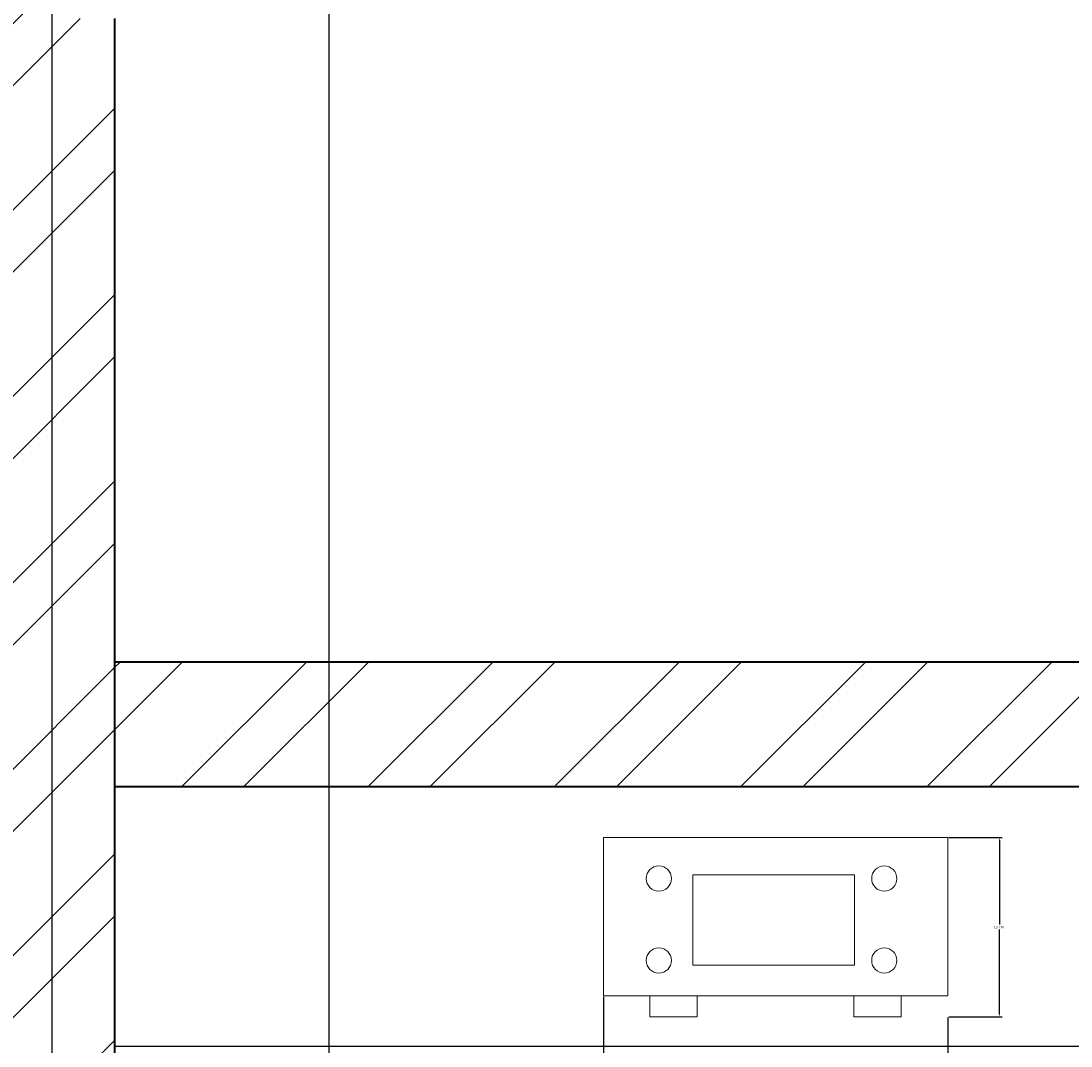
# Model space of a CAD drawing. Units: inches. Extents: x 1601 to 2297, y 1496 to 2631.
# Tile 28 of 57: x 2033 to 2109, y 2067 to 2141. Entities that reach past the tile are written whole.
import ezdxf

# ---------------------------------------------------------------- set-up
doc = ezdxf.new("R2010")
doc.units = ezdxf.units.IN
for name, color, linetype, lineweight in [('A-ANNO-DIMS', 2, 'Continuous', 18), ('A-EQPM', 8, 'Continuous', 18), ('A-WALL', 7, 'Continuous', 40), ('A-WALL-PATT', 215, 'Continuous', 13)]:
    doc.layers.add(name, color=color, linetype=linetype, lineweight=lineweight)
doc.styles.get("Standard").update_dxf_attribs({"font": 'arial.ttf'})
doc.dimstyles.get("Standard").update_dxf_attribs({"dimtxt": 0.18, "dimasz": 0.18, "dimexe": 0.18, "dimexo": 0.0625, "dimgap": 0.09, "dimtad": 0, "dimtih": 1, "dimtoh": 1, "dimdec": 4, "dimzin": 0, "dimdsep": 46, "dimtxsty": 'Standard', "dimcen": 0.09, "dimadec": 0, "dimazin": 0, "dimtfac": 1, "dimtdec": 4, "dimtofl": 0, "dimtmove": 0, "dimatfit": 3, "dimfxl": 1, "dimtolj": 1, "dimtzin": 0, "dimarcsym": 0})

# ---------------------------------------------------------------- blocks, each defined once
blk = doc.blocks.new('COOKTOP-4-BURNER')
for points in [[(0, 12.954), (24.894, 12.954), (24.894, 1.511), (0, 1.511)], [(6.453, 10.253), (18.146, 10.253), (18.146, 3.736), (6.453, 3.736)], [(3.349, 1.511), (6.775, 1.511), (6.775, 0), (3.349, 0)], [(18.089, 1.511), (21.515, 1.511), (21.515, 0), (18.089, 0)], [(18.089, 1.511), (21.515, 1.511), (21.515, 0), (18.089, 0)]]:
    blk.add_lwpolyline(points, close=True)
for centre in [(3.995, 9.987), (20.29, 9.987), (3.995, 4.07), (20.29, 4.07)]:
    blk.add_circle(centre, 0.91)
blk = doc.blocks.new('*D18')
at = {"layer": 'A-ANNO-DIMS', "color": 0, "lineweight": -2, "transparency": 16777216}
for p, q in [((2075.398, 2068.626), (2075.398, 2064.774)), ((2100.291, 2068.626), (2100.291, 2064.774)), ((2075.578, 2064.954), (2086.654, 2064.954)), ((2100.111, 2064.954), (2089.035, 2064.954))]:
    blk.add_line(p, q, dxfattribs=at)
at = {"layer": 'A-ANNO-DIMS', "color": 0, "transparency": 16777216}
for points in [[(2075.578, 2064.984), (2075.578, 2064.924), (2075.398, 2064.954)], [(2100.111, 2064.984), (2100.111, 2064.924), (2100.291, 2064.954)]]:
    blk.add_solid(points, dxfattribs=at)
at = {"layer": 'Defpoints', "color": 0, "transparency": 16777216}
for p in [(2075.398, 2068.688), (2100.291, 2068.688), (2100.291, 2064.954)]:
    blk.add_point(p, dxfattribs=at)
at = {"layer": 'A-ANNO-DIMS', "color": 0, "transparency": 16777216, "insert": (2087.844, 2064.954), "char_height": 0.18, "attachment_point": 5}
blk.add_mtext('\\A1;COOKTOP 25 TYP.', dxfattribs=at)
blk = doc.blocks.new('*D19')
at = {"layer": 'A-ANNO-DIMS', "color": 0, "lineweight": -2, "transparency": 16777216}
for p, q in [((2100.353, 2081.642), (2104.205, 2081.642)), ((2104.025, 2081.462), (2104.025, 2075.347)), ((2104.025, 2068.868), (2104.025, 2074.983)), ((2100.353, 2068.688), (2104.205, 2068.688))]:
    blk.add_line(p, q, dxfattribs=at)
at = {"layer": 'A-ANNO-DIMS', "color": 0, "transparency": 16777216}
for points in [[(2103.995, 2081.462), (2104.055, 2081.462), (2104.025, 2081.642)], [(2103.995, 2068.868), (2104.055, 2068.868), (2104.025, 2068.688)]]:
    blk.add_solid(points, dxfattribs=at)
at = {"layer": 'Defpoints', "color": 0, "transparency": 16777216}
for p in [(2100.291, 2081.642), (2104.025, 2081.642), (2100.291, 2068.688)]:
    blk.add_point(p, dxfattribs=at)
at = {"layer": 'A-ANNO-DIMS', "color": 0, "transparency": 16777216, "insert": (2104.025, 2075.165), "char_height": 0.18, "attachment_point": 5}
blk.add_mtext('\\A1;13 TYP.', dxfattribs=at)
blk = doc.blocks.new('*D37')
at = {"layer": 'A-ANNO-DIMS', "color": 0, "lineweight": -2, "transparency": 16777216}
for p, q in [((2040.1, 2085.325), (2279.267, 2085.325)), ((2279.087, 2085.145), (2279.087, 2076.132)), ((2279.087, 2066.755), (2279.087, 2075.768)), ((2040.1, 2066.575), (2279.267, 2066.575))]:
    blk.add_line(p, q, dxfattribs=at)
at = {"layer": 'A-ANNO-DIMS', "color": 0, "transparency": 16777216}
for points in [[(2279.057, 2085.145), (2279.117, 2085.145), (2279.087, 2085.325)], [(2279.057, 2066.755), (2279.117, 2066.755), (2279.087, 2066.575)]]:
    blk.add_solid(points, dxfattribs=at)
at = {"layer": 'Defpoints', "color": 0, "transparency": 16777216}
for p in [(2040.037, 2085.325), (2279.087, 2085.325), (2040.037, 2066.575)]:
    blk.add_point(p, dxfattribs=at)
at = {"layer": 'A-ANNO-DIMS', "color": 0, "transparency": 16777216, "insert": (2279.087, 2075.95), "char_height": 0.18, "attachment_point": 5}
blk.add_mtext('\\A1;18.75', dxfattribs=at)
blk = doc.blocks.new('*D40')
at = {"layer": 'A-ANNO-DIMS', "color": 0, "lineweight": -2, "transparency": 16777216}
for p, q in [((2035.537, 1986.388), (2035.537, 2581.055)), ((2035.717, 2580.875), (2045.079, 2580.875)), ((2055.371, 2580.875), (2046.009, 2580.875)), ((2055.551, 1986.388), (2055.551, 2581.055))]:
    blk.add_line(p, q, dxfattribs=at)
at = {"layer": 'A-ANNO-DIMS', "color": 0, "transparency": 16777216}
for points in [[(2035.717, 2580.905), (2035.717, 2580.845), (2035.537, 2580.875)], [(2055.371, 2580.905), (2055.371, 2580.845), (2055.551, 2580.875)]]:
    blk.add_solid(points, dxfattribs=at)
at = {"layer": 'Defpoints', "color": 0, "transparency": 16777216}
for p in [(2055.551, 2580.875), (2035.537, 1986.325), (2055.551, 1986.325)]:
    blk.add_point(p, dxfattribs=at)
at = {"layer": 'A-ANNO-DIMS', "color": 0, "transparency": 16777216, "insert": (2045.544, 2580.875), "char_height": 0.18, "attachment_point": 5}
blk.add_mtext('\\A1;20.014', dxfattribs=at)
blk = doc.blocks.new('*D41')
at = {"layer": 'A-ANNO-DIMS', "color": 0, "lineweight": -2, "transparency": 16777216}
for p, q in [((2075.398, 2070.136), (2075.398, 1513.748)), ((2040.037, 2066.513), (2040.037, 1513.748)), ((2040.217, 1513.928), (2057.324, 1513.928)), ((2075.218, 1513.928), (2058.111, 1513.928))]:
    blk.add_line(p, q, dxfattribs=at)
at = {"layer": 'A-ANNO-DIMS', "color": 0, "transparency": 16777216}
for points in [[(2040.217, 1513.958), (2040.217, 1513.898), (2040.037, 1513.928)], [(2075.218, 1513.958), (2075.218, 1513.898), (2075.398, 1513.928)]]:
    blk.add_solid(points, dxfattribs=at)
at = {"layer": 'Defpoints', "color": 0, "transparency": 16777216}
for p in [(2075.398, 2070.199), (2040.037, 2066.575), (2075.398, 1513.928)]:
    blk.add_point(p, dxfattribs=at)
at = {"layer": 'A-ANNO-DIMS', "color": 0, "transparency": 16777216, "insert": (2057.717, 1513.928), "char_height": 0.18, "attachment_point": 5}
blk.add_mtext('\\A1;35.36', dxfattribs=at)

msp = doc.modelspace()

# ---------------------------------------------------------------- hatches: boundary and pattern name
at = {"layer": 'A-WALL-PATT'}
h = msp.add_hatch(dxfattribs=at)
h.set_pattern_fill('ANSI32', color=256)
h.paths.add_polyline_path([(1973.9371, 2211.3254), (1893.0373, 2211.3254), (1893.0373, 2287.8254), (1884.6167, 2287.8254), (1884.6167, 2285.5754), (1884.6167, 2283.3254), (1888.5373, 2283.3254), (1888.5373, 2145.3254), (1695.0373, 2145.3254), (1695.0373, 2173.8724), (1690.5373, 2173.8724), (1686.0373, 2173.8724), (1686.0373, 2136.3254), (1722.5687, 2136.3254), (1722.5687, 2117.4352), (1731.5687, 2117.4352), (1731.5687, 2136.3254), (1893.0373, 2136.3254), (1893.0373, 2202.3254), (1959.0373, 2202.3254), (1959.0373, 2182.1303), (1968.0373, 2182.1303), (1968.0373, 2202.3254), (1973.9371, 2202.3254)])
h.paths.add_polyline_path([(2094.0373, 2274.6364), (2096.4294, 2274.6364), (2096.4294, 2276.8864), (2096.4294, 2279.1364), (2094.0373, 2279.1364), (2094.0373, 2290.8254), (2094.0373, 2295.3254), (2089.5373, 2295.3254), (2089.5373, 2230.8254), (2035.5373, 2230.8254), (2035.5373, 2299.8254), (2031.0373, 2299.8254), (2031.0373, 2211.3254), (2023.0065, 2211.3254), (2023.0065, 2202.3254), (2031.0373, 2202.3254), (2031.0373, 2140.8254), (1968.0373, 2140.8254), (1968.0373, 2145.9106), (1963.5373, 2145.9106), (1959.0373, 2145.9106), (1959.0373, 2116.839), (1963.5373, 2116.839), (1968.0373, 2116.839), (1968.0373, 2131.8254), (2031.0373, 2131.8254), (2031.0373, 2094.3254), (2031.0373, 2085.3254), (2031.0373, 2056.8254), (1968.0373, 2056.8254), (1968.0373, 2070.4947), (1963.5373, 2070.4947), (1959.0373, 2070.4947), (1959.0373, 2040.3029), (1968.0373, 2040.3029), (1968.0373, 2047.8254), (2031.0373, 2047.8254), (2031.0373, 1983.3254), (2031.0373, 1978.8254), (2021.1979, 1978.8254), (2021.1979, 1974.3254), (2031.0373, 1974.3254), (2031.0373, 1954.3528), (2035.5373, 1954.3528), (2035.5373, 1974.3254), (2035.5373, 1981.8254), (2055.5513, 1981.8254), (2055.5513, 1986.3254), (2035.5373, 1986.3254), (2035.5373, 2047.8254), (2040.0373, 2047.8254), (2040.0373, 2085.3254), (2040.0373, 2094.3254), (2040.0373, 2140.8254), (2035.5373, 2140.8254), (2035.5373, 2226.3254), (2089.5373, 2226.3254), (2094.0373, 2226.3254)])
h.paths.add_polyline_path([(2226.0373, 2230.8254), (2134.5373, 2230.8254), (2134.5373, 2233.5437), (2130.0373, 2233.5437), (2130.0373, 2226.3254), (2134.5373, 2226.3254), (2226.0373, 2226.3254)])
h.paths.add_polyline_path([(1807.1169, 1573.5395), (2055.0405, 1573.5395), (2055.0405, 1610.6322), (1807.1169, 1610.6322)], flags=9)
h.paths.add_polyline_path([(1841.1631, 1712.7967), (1870.3957, 1712.7967), (1870.3957, 1731.454), (1841.1631, 1731.454)], flags=9)
h.paths.add_polyline_path([(2144.3862, 1772.185), (2191.0233, 1772.185), (2191.0233, 1790.8423), (2144.3862, 1790.8423)], flags=9)
h.paths.add_polyline_path([(2143.0128, 1827.3312), (2177.9958, 1827.3312), (2177.9958, 1845.9886), (2143.0128, 1845.9886)], flags=9)
h.paths.add_polyline_path([(2041.2439, 1833.5691), (2070.8516, 1833.5691), (2070.8516, 1852.2264), (2041.2439, 1852.2264)], flags=9)
h.paths.add_polyline_path([(2097.2791, 1947.0598), (2134.2061, 1947.0598), (2134.2061, 1965.7171), (2097.2791, 1965.7171)], flags=9)
h.paths.add_polyline_path([(2214.995, 1904.3124), (2214.995, 1942.2899), (2196.3376, 1942.2899), (2196.3376, 1904.3124)], flags=9)
h.paths.add_polyline_path([(2186.6284, 2043.8031), (2219.7935, 2043.8031), (2219.7935, 2062.4605), (2186.6284, 2062.4605)], flags=9)
h.paths.add_polyline_path([(2064.0877, 2031.616), (2097.4949, 2031.616), (2097.4949, 2050.2734), (2064.0877, 2050.2734)], flags=9)
h.paths.add_polyline_path([(1973.1349, 1986.0688), (2008.4009, 1986.0688), (2008.4009, 2004.7261), (1973.1349, 2004.7261)], flags=25)
h.paths.add_polyline_path([(1976.3676, 2106.9635), (2005.7469, 2106.9635), (2005.7469, 2125.6209), (1976.3676, 2125.6209)], flags=25)
h.paths.add_polyline_path([(1991.7852, 2180.4863), (2027.0513, 2180.4863), (2027.0513, 2199.1437), (1991.7852, 2199.1437)], flags=25)
h.paths.add_polyline_path([(2106.1801, 2187.9359), (2152.2101, 2187.9359), (2152.2101, 2206.5932), (2106.1801, 2206.5932)], flags=9)
h.paths.add_polyline_path([(2148.6686, 2262.2542), (2182.318, 2262.2542), (2182.318, 2280.9115), (2148.6686, 2280.9115)], flags=9)
h.paths.add_polyline_path([(2041.6327, 2252.8147), (2071.2405, 2252.8147), (2071.2405, 2271.4721), (2041.6327, 2271.4721)], flags=25)
h.paths.add_polyline_path([(2063.9734, 2375.4265), (2100.9004, 2375.4265), (2100.9004, 2394.0839), (2063.9734, 2394.0839)], flags=9)
h.paths.add_polyline_path([(2216.4955, 2330.9748), (2216.4955, 2370.2654), (2197.8381, 2370.2654), (2197.8381, 2330.9748)], flags=9)
h.paths.add_polyline_path([(2179.1416, 2485.8687), (2212.3067, 2485.8687), (2212.3067, 2504.5261), (2179.1416, 2504.5261)], flags=9)
h.paths.add_polyline_path([(2078.7442, 2471.1516), (2112.1514, 2471.1516), (2112.1514, 2489.809), (2078.7442, 2489.809)], flags=9)
h.paths.add_polyline_path([(1915.9631, 2329.4668), (1952.8902, 2329.4668), (1952.8902, 2348.1241), (1915.9631, 2348.1241)], flags=9)
h.paths.add_polyline_path([(1904.3189, 2499.6709), (1940.4512, 2499.6709), (1940.4512, 2518.3282), (1904.3189, 2518.3282)], flags=9)
h.paths.add_polyline_path([(1892.3665, 2100.4595), (1925.6374, 2100.4595), (1925.6374, 2119.1169), (1892.3665, 2119.1169)], flags=9)
h.paths.add_polyline_path([(1909.2984, 1805.9631), (1946.2254, 1805.9631), (1946.2254, 1824.6205), (1909.2984, 1824.6205)], flags=9)
h.paths.add_polyline_path([(1934.6056, 1658.616), (1970.738, 1658.616), (1970.738, 1677.2733), (1934.6056, 1677.2733)], flags=9)
h.paths.add_polyline_path([(1711.2052, 1789.8902), (1750.0456, 1789.8902), (1750.0456, 1808.5476), (1711.2052, 1808.5476)], flags=9)
h.paths.add_polyline_path([(1742.7874, 1854.6743), (1771.9449, 1854.6743), (1771.9449, 1873.3317), (1742.7874, 1873.3317)], flags=9)
h.paths.add_polyline_path([(1807.3592, 1997.7912), (1850.1116, 1997.7912), (1850.1116, 2016.4486), (1807.3592, 2016.4486)], flags=9)
h.paths.add_polyline_path([(1717.4579, 2237.7844), (1760.2103, 2237.7844), (1760.2103, 2256.4417), (1717.4579, 2256.4417)], flags=25)
h.paths.add_polyline_path([(1780.9285, 2324.0623), (1810.086, 2324.0623), (1810.086, 2342.7197), (1780.9285, 2342.7197)], flags=9)
h.paths.add_polyline_path([(1837.696, 2449.2024), (1866.9286, 2449.2024), (1866.9286, 2467.8598), (1837.696, 2467.8598)], flags=9)
h.paths.add_polyline_path([(1712.7752, 2484.9404), (1751.6156, 2484.9404), (1751.6156, 2503.5977), (1712.7752, 2503.5977)], flags=9)
h = msp.add_hatch(dxfattribs=at)
h.set_pattern_fill('ANSI32', color=256)
h.paths.add_polyline_path([(2230.5373, 1861.8254), (2182.5373, 1861.8254), (2182.5373, 1885.3637), (2178.0373, 1885.3637), (2178.0373, 1861.8254), (2166.0373, 1861.8254), (2134.5373, 1861.8254), (2130.0373, 1861.8254), (2130.0373, 1841.4682), (2126.8833, 1841.4682), (2126.8833, 1836.9682), (2130.0373, 1836.9682), (2130.0373, 1822.7302), (2134.5373, 1822.7302), (2134.5373, 1857.3254), (2166.0373, 1857.3254), (2226.0373, 1857.3254), (2226.0373, 1846.1155), (2230.5373, 1846.1155)])
h.paths.add_polyline_path([(2226.0373, 1797.3254), (2134.5373, 1797.3254), (2134.5373, 1800.6636), (2132.2873, 1800.6636), (2130.0373, 1800.6636), (2130.0373, 1797.3254), (2130.0373, 1792.8254), (2167.7264, 1792.8254), (2226.0373, 1792.8254)])
h.paths.add_polyline_path([(2230.5373, 1822.1155), (2226.0373, 1822.1155), (2226.0373, 1760.8563), (2230.5373, 1760.8563)])
h.paths.add_polyline_path([(2230.5373, 1700.8563), (2226.0373, 1700.8563), (2226.0373, 1644.3254), (2140.2517, 1644.3254), (2140.2517, 1635.3254), (2230.5373, 1635.3254)])
h.paths.add_polyline_path([(2080.2517, 1639.8254), (2080.2517, 1644.3254), (2035.5373, 1644.3254), (2035.5373, 1792.8254), (2094.0373, 1792.8254), (2094.0373, 1797.3254), (2094.0373, 1836.9682), (2097.1057, 1836.9682), (2097.1057, 1839.2182), (2097.1057, 1841.4682), (2094.0373, 1841.4682), (2094.0373, 1862.2276), (2089.5373, 1862.2276), (2089.5373, 1797.3254), (2035.5373, 1797.3254), (2035.5373, 1857.3254), (2035.5373, 1885.0916), (2031.0373, 1885.0916), (2031.0373, 1710.3254), (2012.329, 1710.3254), (2012.329, 1701.3254), (2031.0373, 1701.3254), (2031.0373, 1644.3254), (2031.0373, 1635.3254), (2080.2517, 1635.3254)])
h.paths.add_polyline_path([(1836.0373, 1653.2033), (1842.6171, 1653.2033), (1842.6171, 1657.7033), (1842.6171, 1662.2033), (1831.5373, 1662.2033), (1831.5373, 1764.2033), (1835.3881, 1764.2033), (1835.3881, 1766.4533), (1835.3881, 1768.7033), (1831.5373, 1768.7033), (1827.0373, 1768.7033), (1827.0373, 1662.2033), (1827.0373, 1635.3254), (1836.0373, 1635.3254)])
h.paths.add_polyline_path([(1893.0373, 1701.3254), (1907.193, 1701.3254), (1907.193, 1705.8254), (1907.193, 1710.3254), (1893.0373, 1710.3254), (1893.0373, 1819.8254), (1882.6444, 1819.8254), (1882.6444, 1817.5754), (1882.6444, 1815.3254), (1888.5373, 1815.3254), (1888.5373, 1662.2033), (1884.0373, 1662.2033), (1866.6171, 1662.2033), (1866.6171, 1653.2033), (1882.391, 1653.2033), (1884.0373, 1653.2033), (1884.0373, 1635.3254), (1893.0373, 1635.3254)])
h.paths.add_polyline_path([(1739.3335, 1639.8254), (1739.3335, 1644.3254), (1695.0373, 1644.3254), (1695.0373, 1702.0135), (1690.5373, 1702.0135), (1686.0373, 1702.0135), (1686.0373, 1635.3254), (1739.3335, 1635.3254)])
h.paths.add_polyline_path([(1827.0373, 1644.3254), (1799.3335, 1644.3254), (1799.3335, 1635.3254), (1827.0373, 1635.3254)])
h.paths.add_polyline_path([(1695.0373, 1815.3254), (1849.2759, 1815.3254), (1849.2759, 1819.8254), (1807.5373, 1819.8254), (1807.5373, 1879.8254), (1851.1533, 1879.8254), (1851.1533, 1882.0754), (1851.1533, 1884.3254), (1799.3405, 1884.3254), (1799.3405, 1882.0754), (1799.3405, 1879.8254), (1803.0373, 1879.8254), (1803.0373, 1819.8254), (1695.0373, 1819.8254), (1695.0373, 1835.0458), (1690.5373, 1835.0458), (1686.0373, 1835.0458), (1686.0373, 1766.1753), (1695.0373, 1766.1753)])
h.paths.add_polyline_path([(1775.8157, 1884.3254), (1695.0373, 1884.3254), (1695.0373, 1912.9526), (1690.5373, 1912.9526), (1686.0373, 1912.9526), (1686.0373, 1859.0458), (1695.0373, 1859.0458), (1695.0373, 1879.8254), (1775.8157, 1879.8254)])
h.paths.add_polyline_path([(1893.0373, 2031.3254), (1731.5687, 2031.3254), (1731.5687, 2057.4352), (1722.5687, 2057.4352), (1722.5687, 2031.3254), (1686.0373, 2031.3254), (1686.0373, 1972.9526), (1695.0373, 1972.9526), (1695.0373, 2022.3254), (1888.5373, 2022.3254), (1888.5373, 1884.3254), (1883.4996, 1884.3254), (1883.4996, 1879.8254), (1893.0373, 1879.8254), (1893.0373, 1974.3254), (1976.6199, 1974.3254), (1976.6199, 1978.8254), (1968.0373, 1978.8254), (1968.0373, 1983.3254), (1968.0373, 2008.4756), (1963.5373, 2008.4756), (1959.0373, 2008.4756), (1959.0373, 1983.3254), (1893.0373, 1983.3254)])
h.paths.add_polyline_path([(2230.5373, 2140.4745), (2226.0373, 2140.4745), (2226.0373, 2094.3254), (2040.0373, 2094.3254), (2040.0373, 2085.3254), (2178.0373, 2085.3254), (2178.0373, 2065.6965), (2182.5373, 2065.6965), (2182.5373, 2085.3254), (2226.0373, 2085.3254), (2226.0373, 1986.3254), (2211.2679, 1986.3254), (2211.2679, 1981.8254), (2230.5373, 1981.8254)])
h.paths.add_polyline_path([(2187.6292, 1986.3254), (2182.5373, 1986.3254), (2182.5373, 2029.6965), (2178.0373, 2029.6965), (2178.0373, 1986.3254), (2099.05, 1986.3254), (2099.05, 1981.8254), (2178.0373, 1981.8254), (2178.0373, 1969.3637), (2182.5373, 1969.3637), (2182.5373, 1981.8254), (2187.6292, 1981.8254), (2187.6292, 1984.0754)])
h.paths.add_polyline_path([(1807.1169, 1573.5395), (2055.0405, 1573.5395), (2055.0405, 1610.6322), (1807.1169, 1610.6322)], flags=9)
h.paths.add_polyline_path([(1841.1631, 1712.7967), (1870.3957, 1712.7967), (1870.3957, 1731.454), (1841.1631, 1731.454)], flags=9)
h.paths.add_polyline_path([(2144.3862, 1772.185), (2191.0233, 1772.185), (2191.0233, 1790.8423), (2144.3862, 1790.8423)], flags=9)
h.paths.add_polyline_path([(2143.0128, 1827.3312), (2177.9958, 1827.3312), (2177.9958, 1845.9886), (2143.0128, 1845.9886)], flags=25)
h.paths.add_polyline_path([(2041.2439, 1833.5691), (2070.8516, 1833.5691), (2070.8516, 1852.2264), (2041.2439, 1852.2264)], flags=25)
h.paths.add_polyline_path([(2097.2791, 1947.0598), (2134.2061, 1947.0598), (2134.2061, 1965.7171), (2097.2791, 1965.7171)], flags=9)
h.paths.add_polyline_path([(2214.995, 1904.3124), (2214.995, 1942.2899), (2196.3376, 1942.2899), (2196.3376, 1904.3124)], flags=9)
h.paths.add_polyline_path([(2186.6284, 2043.8031), (2219.7935, 2043.8031), (2219.7935, 2062.4605), (2186.6284, 2062.4605)], flags=25)
h.paths.add_polyline_path([(2064.0877, 2031.616), (2097.4949, 2031.616), (2097.4949, 2050.2734), (2064.0877, 2050.2734)], flags=25)
h.paths.add_polyline_path([(1973.1349, 1986.0688), (2008.4009, 1986.0688), (2008.4009, 2004.7261), (1973.1349, 2004.7261)], flags=9)
h.paths.add_polyline_path([(1976.3676, 2106.9635), (2005.7469, 2106.9635), (2005.7469, 2125.6209), (1976.3676, 2125.6209)], flags=9)
h.paths.add_polyline_path([(1991.7852, 2180.4863), (2027.0513, 2180.4863), (2027.0513, 2199.1437), (1991.7852, 2199.1437)], flags=9)
h.paths.add_polyline_path([(2106.1801, 2187.9359), (2152.2101, 2187.9359), (2152.2101, 2206.5932), (2106.1801, 2206.5932)], flags=9)
h.paths.add_polyline_path([(2148.6686, 2262.2542), (2182.318, 2262.2542), (2182.318, 2280.9115), (2148.6686, 2280.9115)], flags=9)
h.paths.add_polyline_path([(2041.6327, 2252.8147), (2071.2405, 2252.8147), (2071.2405, 2271.4721), (2041.6327, 2271.4721)], flags=9)
h.paths.add_polyline_path([(2063.9734, 2375.4265), (2100.9004, 2375.4265), (2100.9004, 2394.0839), (2063.9734, 2394.0839)], flags=9)
h.paths.add_polyline_path([(2216.4955, 2330.9748), (2216.4955, 2370.2654), (2197.8381, 2370.2654), (2197.8381, 2330.9748)], flags=9)
h.paths.add_polyline_path([(2179.1416, 2485.8687), (2212.3067, 2485.8687), (2212.3067, 2504.5261), (2179.1416, 2504.5261)], flags=9)
h.paths.add_polyline_path([(2078.7442, 2471.1516), (2112.1514, 2471.1516), (2112.1514, 2489.809), (2078.7442, 2489.809)], flags=9)
h.paths.add_polyline_path([(1915.9631, 2329.4668), (1952.8902, 2329.4668), (1952.8902, 2348.1241), (1915.9631, 2348.1241)], flags=9)
h.paths.add_polyline_path([(1904.3189, 2499.6709), (1940.4512, 2499.6709), (1940.4512, 2518.3282), (1904.3189, 2518.3282)], flags=9)
h.paths.add_polyline_path([(1892.3665, 2100.4595), (1925.6374, 2100.4595), (1925.6374, 2119.1169), (1892.3665, 2119.1169)], flags=9)
h.paths.add_polyline_path([(1909.2984, 1805.9631), (1946.2254, 1805.9631), (1946.2254, 1824.6205), (1909.2984, 1824.6205)], flags=9)
h.paths.add_polyline_path([(1934.6056, 1658.616), (1970.738, 1658.616), (1970.738, 1677.2733), (1934.6056, 1677.2733)], flags=9)
h.paths.add_polyline_path([(1711.2052, 1789.8902), (1750.0456, 1789.8902), (1750.0456, 1808.5476), (1711.2052, 1808.5476)], flags=25)
h.paths.add_polyline_path([(1742.7874, 1854.6743), (1771.9449, 1854.6743), (1771.9449, 1873.3317), (1742.7874, 1873.3317)], flags=25)
h.paths.add_polyline_path([(1807.3592, 1997.7912), (1850.1116, 1997.7912), (1850.1116, 2016.4486), (1807.3592, 2016.4486)], flags=25)
h.paths.add_polyline_path([(1717.4579, 2237.7844), (1760.2103, 2237.7844), (1760.2103, 2256.4417), (1717.4579, 2256.4417)], flags=9)
h.paths.add_polyline_path([(1780.9285, 2324.0623), (1810.086, 2324.0623), (1810.086, 2342.7197), (1780.9285, 2342.7197)], flags=9)
h.paths.add_polyline_path([(1837.696, 2449.2024), (1866.9286, 2449.2024), (1866.9286, 2467.8598), (1837.696, 2467.8598)], flags=9)
h.paths.add_polyline_path([(1712.7752, 2484.9404), (1751.6156, 2484.9404), (1751.6156, 2503.5977), (1712.7752, 2503.5977)], flags=9)

# ---------------------------------------------------------------- linework, layer by layer
at = {"layer": 'A-WALL'}
for p, q in [((2040.0373, 2140.8254), (2040.0373, 2094.3254)), ((2226.0373, 2094.3254), (2040.0373, 2094.3254)), ((2040.0373, 2094.3254), (2040.0373, 2085.3254)), ((2040.0373, 2085.3254), (2178.0373, 2085.3254)), ((2040.0373, 2085.3254), (2040.0373, 2047.8254)), ((2040.0373, 2085.3254), (2178.0373, 2085.3254))]:
    msp.add_line(p, q, dxfattribs=at)

# ---------------------------------------------------------------- block references
at = {"layer": 'A-EQPM'}
msp.add_blockref('COOKTOP-4-BURNER', (2075.3972, 2068.6882), dxfattribs=at)

# ---------------------------------------------------------------- dimensions: what is measured, and where the dimension line sits
at = {"layer": 'A-ANNO-DIMS'}
for base, p1, p2, override, picture, middle in [((2055.5513, 2580.8754), (2035.5373, 1986.3254), (2055.5513, 1986.3254), {"dimdec": 3, "dimlfac": 1, "dimrnd": 0, "dimzin": 0, "dimdsep": 46, "dimlunit": 2}, '*D40', (2045.5443, 2580.8754)), ((2075.3977, 1513.9279), (2040.0373, 2066.5754), (2075.3977, 2070.1988), {"dimdec": 2, "dimlfac": 1, "dimrnd": 0, "dimzin": 0, "dimdsep": 46, "dimlunit": 2}, '*D41', (2057.7175, 1513.9279))]:
    dim = msp.add_linear_dim(base=base, p1=p1, p2=p2, dimstyle='Standard', override=override, dxfattribs=at)
    dim.commit()
    dim.dimension.update_dxf_attribs({"geometry": picture, "text_midpoint": middle})
dim = msp.add_linear_dim(base=(2279.0873, 2085.3254), p1=(2040.0373, 2066.5754), p2=(2040.0373, 2085.3254), angle=90, dimstyle='Standard', override={"dimdec": 2, "dimlfac": 1, "dimrnd": 0, "dimzin": 0, "dimdsep": 46, "dimlunit": 2}, dxfattribs=at)
dim.commit()
dim.dimension.update_dxf_attribs({"geometry": '*D37', "text_midpoint": (2279.0873, 2075.9504)})
dim = msp.add_linear_dim(base=(2104.0249, 2081.6421), p1=(2100.2909, 2068.688), p2=(2100.2909, 2081.6421), angle=90, text='<> TYP.', dimstyle='Standard', override={"dimdec": 0, "dimlfac": 1, "dimrnd": 0, "dimzin": 0, "dimdsep": 46, "dimlunit": 2}, dxfattribs=at)
dim.commit()
dim.dimension.update_dxf_attribs({"geometry": '*D19', "text_midpoint": (2104.0249, 2075.1651)})
dim = msp.add_linear_dim(base=(2100.2909, 2064.954), p1=(2075.3977, 2068.688), p2=(2100.2909, 2068.688), text='COOKTOP <> TYP.', dimstyle='Standard', override={"dimdec": 0, "dimlfac": 1, "dimrnd": 0, "dimzin": 0, "dimdsep": 46, "dimlunit": 2}, dxfattribs=at)
dim.commit()
dim.dimension.update_dxf_attribs({"geometry": '*D18', "text_midpoint": (2087.8443, 2064.954)})

doc.saveas('drawing.dxf')
